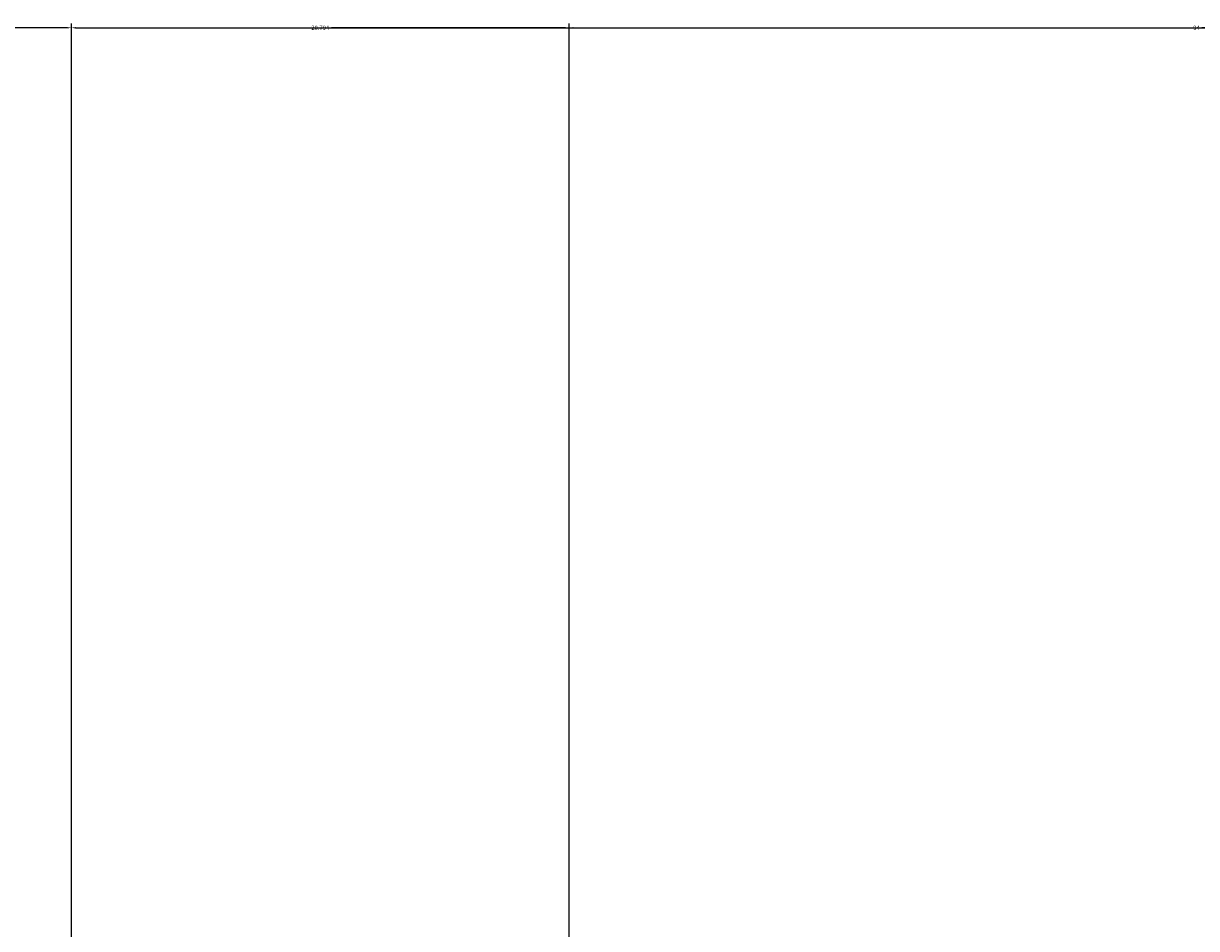
# Model space of a CAD drawing. Units: feet. Extents: x 105 to 1094, y -88 to 588.
# Tile 53 of 59: x 551 to 600, y 551 to 588. Entities that reach past the tile are written whole.
import ezdxf

# ---------------------------------------------------------------- set-up
doc = ezdxf.new("R2010")
doc.units = ezdxf.units.FT
doc.header["$MEASUREMENT"] = 0
doc.layers.add('A-ANNO-DIMS', color=2, linetype='Continuous', lineweight=18)
doc.styles.get("Standard").update_dxf_attribs({"font": 'arial.ttf'})
doc.dimstyles.get("Standard").update_dxf_attribs({"dimtxt": 0.18, "dimasz": 0.18, "dimexe": 0.18, "dimexo": 0.0625, "dimgap": 0.09, "dimtad": 0, "dimtih": 1, "dimtoh": 1, "dimdec": 4, "dimzin": 0, "dimdsep": 46, "dimtxsty": 'Standard', "dimcen": 0.09, "dimadec": 0, "dimazin": 0, "dimtfac": 1, "dimtdec": 4, "dimtofl": 0, "dimtmove": 0, "dimatfit": 3, "dimfxl": 1, "dimtolj": 1, "dimtzin": 0, "dimarcsym": 0})

# ---------------------------------------------------------------- blocks, each defined once
blk = doc.blocks.new('*D25')
at = {"layer": 'A-ANNO-DIMS', "color": 0, "lineweight": -2, "transparency": 16777216}
for p, q in [((438.688, 527.144), (438.688, 588.311)), ((438.868, 588.131), (495.408, 588.131)), ((552.508, 588.131), (495.968, 588.131)), ((552.688, 471.144), (552.688, 588.311))]:
    blk.add_line(p, q, dxfattribs=at)
at = {"layer": 'A-ANNO-DIMS', "color": 0, "transparency": 16777216}
for points in [[(438.868, 588.161), (438.868, 588.101), (438.688, 588.131)], [(552.508, 588.161), (552.508, 588.101), (552.688, 588.131)]]:
    blk.add_solid(points, dxfattribs=at)
at = {"layer": 'Defpoints', "color": 0, "transparency": 16777216}
for p in [(552.688, 588.131), (438.688, 527.081), (552.688, 471.081)]:
    blk.add_point(p, dxfattribs=at)
at = {"layer": 'A-ANNO-DIMS', "color": 0, "transparency": 16777216, "insert": (495.688, 588.131), "char_height": 0.18, "attachment_point": 5}
blk.add_mtext('\\A1;114', dxfattribs=at)
blk = doc.blocks.new('*D26')
at = {"layer": 'A-ANNO-DIMS', "color": 0, "lineweight": -2, "transparency": 16777216}
for p, q in [((552.688, 471.144), (552.688, 588.311)), ((552.868, 588.131), (599.47, 588.131)), ((646.508, 588.131), (599.907, 588.131)), ((646.688, 471.144), (646.688, 588.311))]:
    blk.add_line(p, q, dxfattribs=at)
at = {"layer": 'A-ANNO-DIMS', "color": 0, "transparency": 16777216}
for points in [[(552.868, 588.161), (552.868, 588.101), (552.688, 588.131)], [(646.508, 588.161), (646.508, 588.101), (646.688, 588.131)]]:
    blk.add_solid(points, dxfattribs=at)
at = {"layer": 'Defpoints', "color": 0, "transparency": 16777216}
for p in [(646.688, 588.131), (552.688, 471.081), (646.688, 471.081)]:
    blk.add_point(p, dxfattribs=at)
at = {"layer": 'A-ANNO-DIMS', "color": 0, "transparency": 16777216, "insert": (599.688, 588.131), "char_height": 0.18, "attachment_point": 5}
blk.add_mtext('\\A1;94', dxfattribs=at)
blk = doc.blocks.new('*D47')
at = {"layer": 'A-ANNO-DIMS', "color": 0, "lineweight": -2, "transparency": 16777216}
for p, q in [((552.688, 441.144), (552.688, 588.311)), ((552.868, 588.131), (562.621, 588.131)), ((573.303, 588.131), (563.55, 588.131)), ((573.483, 441.144), (573.483, 588.311))]:
    blk.add_line(p, q, dxfattribs=at)
at = {"layer": 'A-ANNO-DIMS', "color": 0, "transparency": 16777216}
for points in [[(552.868, 588.161), (552.868, 588.101), (552.688, 588.131)], [(573.303, 588.161), (573.303, 588.101), (573.483, 588.131)]]:
    blk.add_solid(points, dxfattribs=at)
at = {"layer": 'Defpoints', "color": 0, "transparency": 16777216}
for p in [(573.483, 588.131), (552.688, 441.081), (573.483, 441.081)]:
    blk.add_point(p, dxfattribs=at)
at = {"layer": 'A-ANNO-DIMS', "color": 0, "transparency": 16777216, "insert": (563.085, 588.131), "char_height": 0.18, "attachment_point": 5}
blk.add_mtext('\\A1;20.794', dxfattribs=at)
blk = doc.blocks.new('*D48')
at = {"layer": 'A-ANNO-DIMS', "color": 0, "lineweight": -2, "transparency": 16777216}
for p, q in [((573.483, 441.144), (573.483, 588.311)), ((573.663, 588.131), (603.263, 588.131)), ((633.303, 588.131), (603.702, 588.131)), ((633.483, 441.144), (633.483, 588.311))]:
    blk.add_line(p, q, dxfattribs=at)
at = {"layer": 'A-ANNO-DIMS', "color": 0, "transparency": 16777216}
for points in [[(573.663, 588.161), (573.663, 588.101), (573.483, 588.131)], [(633.303, 588.161), (633.303, 588.101), (633.483, 588.131)]]:
    blk.add_solid(points, dxfattribs=at)
at = {"layer": 'Defpoints', "color": 0, "transparency": 16777216}
for p in [(633.483, 588.131), (573.483, 441.081), (633.483, 441.081)]:
    blk.add_point(p, dxfattribs=at)
at = {"layer": 'A-ANNO-DIMS', "color": 0, "transparency": 16777216, "insert": (603.483, 588.131), "char_height": 0.18, "attachment_point": 5}
blk.add_mtext('\\A1;60', dxfattribs=at)

msp = doc.modelspace()

# ---------------------------------------------------------------- dimensions: what is measured, and where the dimension line sits
at = {"layer": 'A-ANNO-DIMS'}
for base, p1, p2, override, picture, middle in [((552.6883, 588.1312), (438.6883, 527.0812), (552.6883, 471.0812), {"dimdec": 0, "dimlfac": 1, "dimrnd": 0, "dimzin": 0, "dimdsep": 46, "dimlunit": 2}, '*D25', (495.6883, 588.1312)), ((646.6883, 588.1312), (552.6883, 471.0812), (646.6883, 471.0812), {"dimdec": 0, "dimlfac": 1, "dimrnd": 0, "dimzin": 0, "dimdsep": 46, "dimlunit": 2}, '*D26', (599.6883, 588.1312)), ((573.4826, 588.1312), (552.6883, 441.0812), (573.4826, 441.0812), {"dimdec": 3, "dimlfac": 1, "dimrnd": 0, "dimzin": 0, "dimdsep": 46, "dimlunit": 2}, '*D47', (563.0854, 588.1312)), ((633.4826, 588.1312), (573.4826, 441.0812), (633.4826, 441.0812), {"dimdec": 0, "dimlfac": 1, "dimrnd": 0, "dimzin": 0, "dimdsep": 46, "dimlunit": 2}, '*D48', (603.4826, 588.1312))]:
    dim = msp.add_linear_dim(base=base, p1=p1, p2=p2, dimstyle='Standard', override=override, dxfattribs=at)
    dim.commit()
    dim.dimension.update_dxf_attribs({"geometry": picture, "text_midpoint": middle})

doc.saveas('drawing.dxf')
